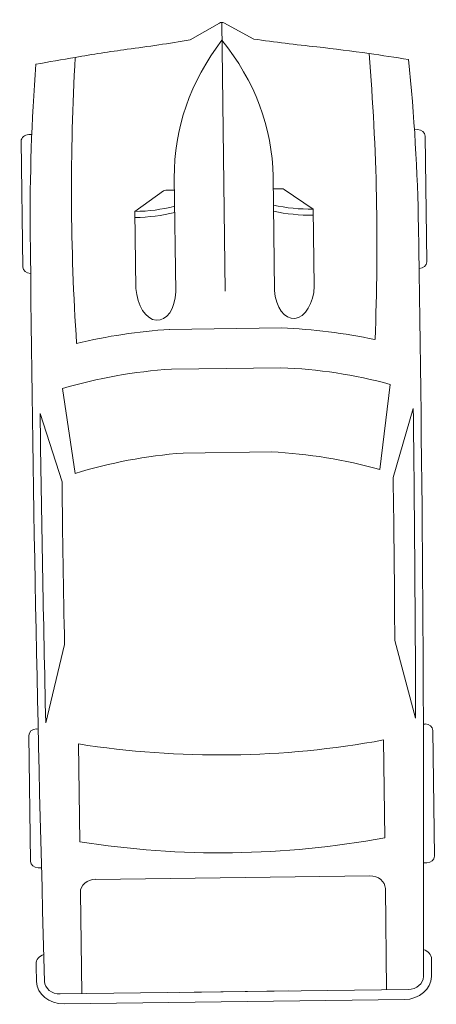
# Model space of a CAD drawing. Units: inches. Extents: x -1085 to 1941, y 1514 to 2348.
# Tile 6 of 9: x 689 to 769, y 1682 to 1872. Entities that reach past the tile are written whole.
import ezdxf

# ---------------------------------------------------------------- set-up
doc = ezdxf.new("R2010")
doc.units = ezdxf.units.IN
doc.layers.add('C-PRKG-VEHS', color=8, linetype='Continuous', lineweight=13)

# ---------------------------------------------------------------- blocks, each defined once
blk = doc.blocks.new('*U28')
for p, q in [((1182.5, 987.8), (567.7, 987.8)), ((3472.1, 987.8), (4086.9, 987.8)), ((536, 950.2), (536, 935.5)), ((1214.1, 949.7), (1214.1, 950.2)), ((3440.5, 941.7), (3440.5, 950.2)), ((4118.5, 950.2), (4118.5, 934.1)), ((2234.8, 809.5), (1898.9, 912.4)), ((3411.6, 904.3), (3029.9, 807.2)), ((4736.4, -850.9), (4736.4, 850.9)), ((4785.3, -832.1), (4785.3, 832.1)), ((1778.8, 801), (2194.7, 745.5)), ((3515.9, 745.5), (3994.1, 745.5)), ((4736.4, 745.5), (4242, 745.5)), ((4178.7, 670.3), (4178.7, -670.3)), ((819.6, 295.3), (917.7, 436.1)), ((917.7, 436.1), (1293.8, 436.1)), ((756.2, 241.4), (1312.8, 241.4)), ((815.9, 241.4), (815.9, 283.3)), ((1496.5, -273.7), (1496.5, 273.7)), ((1690.4, -267.4), (1690.4, 267.4)), ((4736.4, -267.4), (4736.4, 267.4)), ((2101.5, 215.8), (2101.5, -215.8)), ((83, 155.7), (2.6, 10.3)), ((0, 0), (1312.8, 0)), ((2.6, -10.3), (83, -155.7)), ((756.2, -241.4), (1312.8, -241.4)), ((815.9, -241.4), (815.9, -283.3)), ((819.6, -295.3), (917.7, -436.1)), ((917.7, -436.1), (1293.8, -436.1)), ((2194.7, -745.5), (1778.8, -801)), ((3994.1, -745.5), (3515.9, -745.5)), ((4242, -745.5), (4736.4, -745.5)), ((2234.8, -809.5), (1898.9, -912.4)), ((3411.6, -904.3), (3029.9, -807.2)), ((536, -950.2), (536, -935.5)), ((1214.1, -949.7), (1214.1, -950.2)), ((3440.5, -941.7), (3440.5, -950.2)), ((4118.5, -950.2), (4118.5, -934.1)), ((1182.5, -987.8), (567.7, -987.8)), ((3472.1, -987.8), (4086.9, -987.8))]:
    blk.add_line(p, q)
for centre, major_axis, ratio, start_param, end_param in [((567.7, 950.2), (0, -37.6), 0.842304, 3.141593, 4.712389), ((1182.5, 950.2), (0, 37.6), 0.842304, -1.570796, 0), ((3472.1, 950.2), (0, -37.6), 0.842304, 3.141593, 4.712389), ((4086.9, 950.2), (0, 37.6), 0.842304, -1.570796, 0), ((4588, 910.3), (0, 56.4), 0.842304, -0.013017, 1.249894), ((1637.8, -268131.5), (0, 269121), 0.842304, -0.013397, -0.013017), ((4673.1, 832.1), (0, -133.3), 0.842304, 1.570796, 3.128196), ((1046.3, -12467.9), (0, 13417.1), 0.842304, 0.00281, 0.075598), ((1637.8, -268112.7), (0, 269062.9), 0.842304, -0.013397, 0.002797), ((4673.1, 850.9), (0, -75.2), 0.842304, 1.570796, 3.128196), ((6757.2, -699.1), (0, 7958), 0.842304, 1.367076, 1.39176), ((1637.8, -268112.7), (0, -269025.3), 0.842304, 3.133765, 3.140441), ((3436.4, 136.8), (0, 2077), 0.842304, 1.245306, 1.50788), ((2433, -93125.4), (0, -93935.2), 0.842304, 3.134049, 3.144098), ((951.8, -15086.6), (0, -15832.5), 0.842304, 3.096046, 3.200911), ((3413.8, 136.8), (0, -2280.3), 0.842304, 4.449482, 4.652344), ((3799.7, 71.1), (0, -2021.3), 0.842304, 4.372215, 4.640744), ((433.9, 0), (0, 3734.3), 0.842304, 4.511394, 4.913384), ((912, 0), (0, 3734.3), 0.842304, 4.511394, 4.913384), ((4242, 670.3), (0, 75.2), 0.842304, 0, 1.570796), ((6583, -699.1), (0, -7754.7), 0.842304, 4.528606, 4.561838), ((-5194.2, 1330.9), (0, -6374.4), 0.842304, 1.385369, 1.434372), ((331.1, 432), (0, 696.4), 0.842304, 4.435146, 4.718221), ((360.7, 432), (0, 696.4), 0.842304, 4.435146, 4.718221), ((1290.1, 338.8), (161, -9.1), 0.603834, -1.395552, 1.581315), ((831.8, 283.3), (0, 18.8), 0.842304, 0.879714, 1.570796), ((756.2, -1185.2), (0, 1426.7), 0.842304, 0, 0.590319), ((15.8, 0), (0, -18.8), 0.842304, 4.131459, 5.293319), ((756.2, 1185.2), (0, 1426.7), 0.842304, 2.551274, 3.141593), ((-5194.2, -1330.9), (0, 6374.4), 0.842304, -1.434372, -1.385369), ((3799.7, -71.1), (0, -2021.3), 0.842304, -1.499151, -1.230623), ((831.8, -283.3), (0, -18.8), 0.842304, 4.712389, 5.403472), ((331.1, -432), (0, -696.4), 0.842304, 1.564964, 1.848039), ((360.7, -432), (0, -696.4), 0.842304, 1.564964, 1.848039), ((3413.8, -136.8), (0, -2280.3), 0.842304, -1.510751, -1.307889), ((3436.4, -136.8), (0, -2077), 0.842304, -1.50788, -1.245306), ((6583, 699.1), (0, 7754.7), 0.842304, 1.721348, 1.754579), ((4242, -670.3), (0, -75.2), 0.842304, 4.712389, 6.283185), ((6757.2, 699.1), (0, 7958), 0.842304, 1.749832, 1.774517), ((951.8, 15086.6), (0, -15832.5), 0.842304, -0.059319, 0.045547), ((2433, 93125.4), (0, -93935.2), 0.842304, -0.002505, 0.007544), ((4673.1, -850.9), (0, 75.2), 0.842304, 3.15499, 4.712389), ((4673.1, -832.1), (0, -133.3), 0.842304, 0.013397, 1.570796), ((1046.3, 12467.9), (0, -13417.1), 0.842304, -0.075598, -0.00281), ((1637.8, 268112.7), (0, -269025.3), 0.842304, 0.001152, 0.007828), ((567.7, -950.2), (0, 37.6), 0.842304, 1.570796, 3.141593), ((1637.8, 268112.7), (0, 269062.9), 0.842304, 3.138796, 3.15499), ((1182.5, -950.2), (0, -37.6), 0.842304, 0, 1.570796), ((3472.1, -950.2), (0, -37.6), 0.842304, -1.570796, 0), ((4086.9, -950.2), (0, 37.6), 0.842304, 3.141593, 4.712389), ((4588, -910.3), (0, -56.4), 0.842304, -1.249894, 0.013017), ((1637.8, 268131.5), (0, 269121), 0.842304, 3.15461, 3.15499)]:
    blk.add_ellipse(centre, major_axis=major_axis, ratio=ratio, start_param=start_param, end_param=end_param)
at = {"extrusion": (0, 0, -1)}
blk.add_ellipse((1290.1, -338.8), major_axis=(161, 9.1), ratio=0.603834, start_param=-1.395552, end_param=1.581315, dxfattribs=at)

msp = doc.modelspace()

# ---------------------------------------------------------------- block references
at = {"layer": 'C-PRKG-VEHS', "xscale": 0.0393700787401575, "yscale": 0.0393700787401575, "zscale": 0.0393700787401575, "rotation": 270.7362034403327}
msp.add_blockref('*U28', (727.7086, 1871.2556), dxfattribs=at)

doc.saveas('drawing.dxf')
